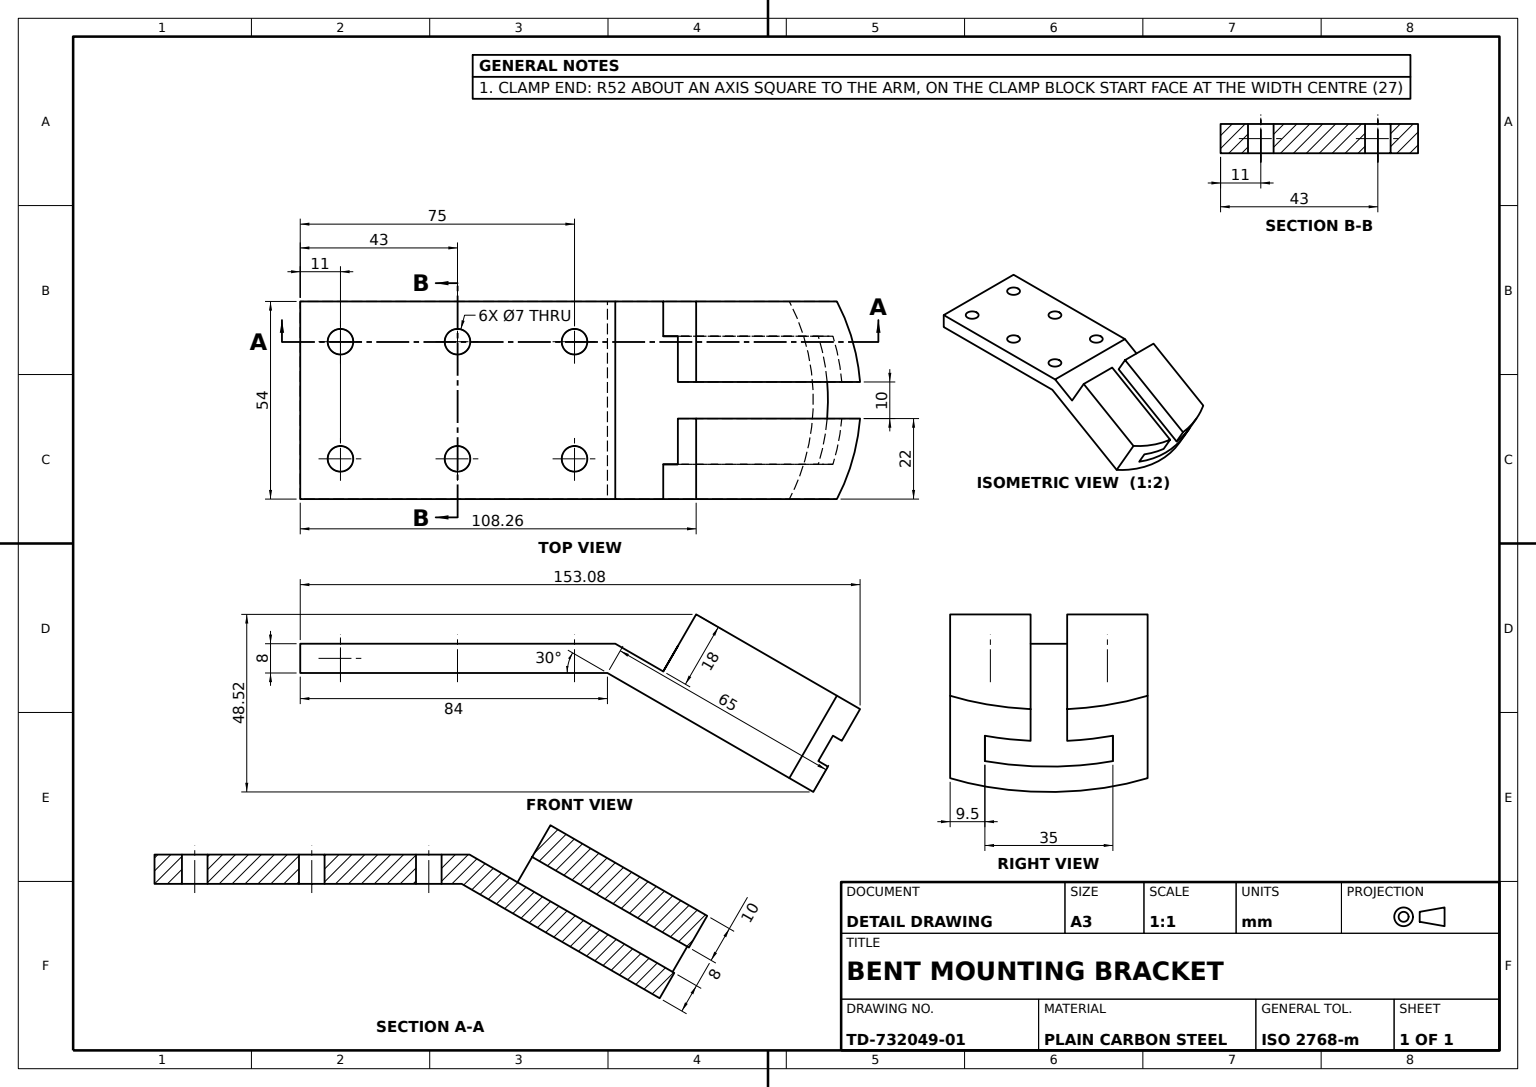
from build123d import *

# Parameters (mm, degrees)
BRACKET_BODY_DEPTH        = 27
CLAMP_SLOT_DEPTH          = 54
CLAMP_END_TRIM_DEPTH      = 54
MOUNTING_HOLES_SKETCH_R   = 3.5
MOUNTING_HOLES_6X_7_DEPTH = 54


with BuildPart() as part:
    # Bracket Profile Sketch → Bracket Body (new, symmetric)
    with BuildSketch(Plane.XY):
        Polygon((108.258330249, 16.016660498), (99.258330249, 0.42820323), (86.143593539, 8), (0, 8), (0, 0), (84, 0), (140.291651246, -32.5), (153.291651246, -9.983339502), align=None)
    extrude(amount=BRACKET_BODY_DEPTH, both=True)

    # Clamp Slot Sketch → Clamp Slot (cut)
    with BuildSketch(Plane(origin=(119.291651246, -68.873066959, 0), x_dir=(0, 0, -1), z_dir=(0.8660254037844386, -0.5000000000000001, 0))):
        Polygon((-17.5, 50), (17.5, 50), (17.5, 58), (5, 58), (5, 68), (-5, 68), (-5, 58), (-17.5, 58), align=None)
    extrude(amount=-CLAMP_SLOT_DEPTH, mode=Mode.SUBTRACT)

    # Clamp End Trim Sketch → Clamp End Trim (cut)
    with BuildSketch(Plane(origin=(34, 58.889727457, 0), x_dir=(0.8660254037844384, -0.5000000000000007, 0), z_dir=(0.5000000000000006, 0.8660254037844383, 0))):
        with BuildLine():
            Line((130.187106004, 27), (186.710578253, 27))
            Line((186.710578253, 27), (186.710578253, -27))
            Line((186.710578253, -27), (130.187106004, -27))
            ThreePointArc((130.187106004, -27), (137.746133918, 0), (130.187106004, 27))
        make_face()
    extrude(amount=-CLAMP_END_TRIM_DEPTH, mode=Mode.SUBTRACT)

    # Mounting Holes Sketch → Mounting Holes 6xØ7 (cut)
    with BuildSketch(Plane(origin=(0, 8, 0), x_dir=(1, 0, 0), z_dir=(0, 1, 0))):
        with Locations(Location((11, 16, 0), (0, 0, 270))):
            Circle(MOUNTING_HOLES_SKETCH_R)
        with Locations(Location((43, 16, 0), (0, 0, 270))):
            Circle(MOUNTING_HOLES_SKETCH_R)
        with Locations(Location((75, 16, 0), (0, 0, 270))):
            Circle(MOUNTING_HOLES_SKETCH_R)
        with Locations(Location((11, -16, 0), (0, 0, 270))):
            Circle(MOUNTING_HOLES_SKETCH_R)
        with Locations(Location((43, -16, 0), (0, 0, 270))):
            Circle(MOUNTING_HOLES_SKETCH_R)
        with Locations(Location((75, -16, 0), (0, 0, 270))):
            Circle(MOUNTING_HOLES_SKETCH_R)
    extrude(amount=-MOUNTING_HOLES_6X_7_DEPTH, mode=Mode.SUBTRACT)


solid = part.part
